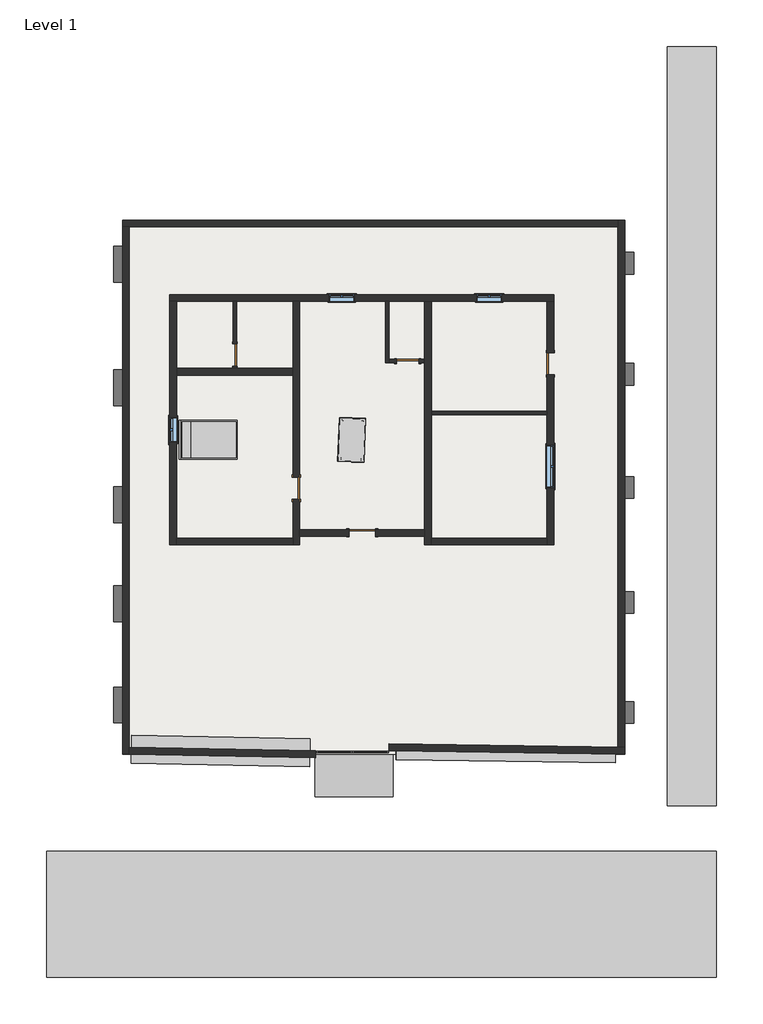
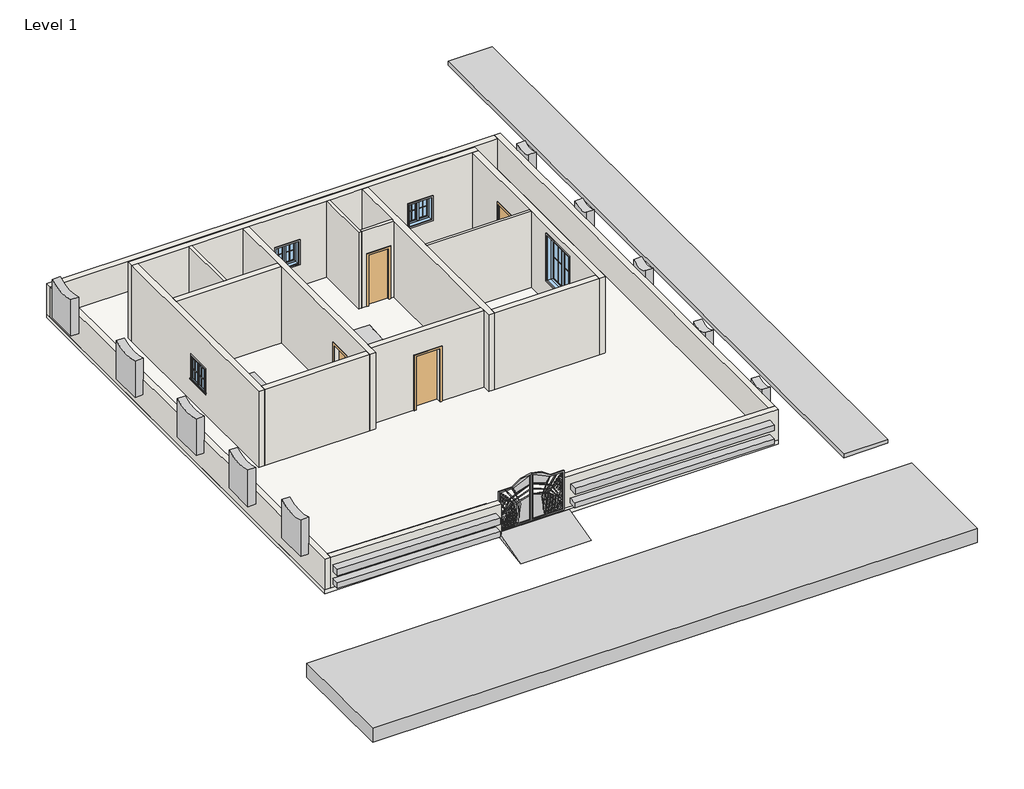
# One storey, incomplete: 24 proxies, 18 walls, 5 doors, 5 windows, 2 furniture elements, 1 slab.
"""IFC4 building model written with IfcOpenShell, lengths in millimetres."""

from ifc_helpers import new_model, si_unit, frame, origin, origin_with_axes, place, context, project, spatial, polyline, outline, extrude, faceted_brep, transform, mapped, element, save
from components import generic_models_6bc30956, generic_models_1_generic_models_1_9ac678b9, generic_models_2_generic_models_2_96ab2cd9, generic_models_4_generic_models_4_b5ce0ccc, generic_models_5_generic_models_5_faea7b41, generic_models_6_generic_models_6_873e410b, generic_models_7_generic_models_7_fbfc4c3c, generic_models_8_generic_models_8_d6955511, muntin_pattern_2x2_muntin_pattern_2x2_b3fe6957, muntin_pattern_2x2_muntin_pattern_2x2_3e0ecaf2, muntin_pattern_2x2_muntin_pattern_2x2_bff912c5, muntin_pattern_2x2_muntin_pattern_2x2_c2194282, trim_window_exterior_flat_with_sill_41619996, trim_window_exterior_flat_with_sill_e04b3088, trim_window_interior_flat_picture_frame_51c85655, trim_window_interior_flat_picture_frame_2a7685fe, door_d8f5dbb5, door_f2b275c1, door_85036156, door_0ca8825f, bed_17739_bed_17739_15c61121, dining_table_14755_dining_table_14755_d89cb775, window_aa618e30, window_339605e1, window_9ac97e1a

model = new_model("IFC4")

# Units and contexts
model_context = context("Model", 3, world=origin())
ifc_project = project(units=[si_unit("LENGTHUNIT", "METRE", prefix="MILLI")], contexts=[model_context])

# Site, building, storey
site = spatial("IfcSite", under=ifc_project)
building = spatial("IfcBuilding", under=site)
storey = spatial("IfcBuildingStorey", under=building, Name="Level 1", Elevation=0.0)

# Proxies
placement = place(None, origin())
generic_models_shape = generic_models_6bc30956(model_context)
element("IfcBuildingElementProxy", 1, Name="Generic Models", at=placement, inside=storey, context=model_context, shape_type="MappedRepresentation", body=[
    mapped(generic_models_shape, transform((-1300.5953031, -8339.7479738, 0.0), x_axis=(1.0, 0.0, 0.0), y_axis=(0.0, 1.0, 0.0), z_axis=(0.0, 0.0, 1.0))),
])
generic_models_1_generic_models_1_shape = generic_models_1_generic_models_1_9ac678b9(model_context)
element("IfcBuildingElementProxy", 2, Name="Generic Models 1 : Generic Models 1", ObjectType="Generic Models 1 : Generic Models 1", at=placement, inside=storey, context=model_context, shape_type="MappedRepresentation", body=[
    mapped(generic_models_1_generic_models_1_shape, transform((0.0, 0.0, 0.0), x_axis=(1.0, 0.0, 0.0), y_axis=(0.0, 1.0, 0.0), z_axis=(0.0, 0.0, 1.0))),
])
generic_models_2_generic_models_2_shape = generic_models_2_generic_models_2_96ab2cd9(model_context)
element("IfcBuildingElementProxy", 3, Name="Generic Models 2 : Generic Models 2", ObjectType="Generic Models 2 : Generic Models 2", at=placement, inside=storey, context=model_context, shape_type="MappedRepresentation", body=[
    mapped(generic_models_2_generic_models_2_shape, transform((0.0, 0.0, 0.0), x_axis=(1.0, 0.0, 0.0), y_axis=(0.0, 1.0, 0.0), z_axis=(0.0, 0.0, 1.0))),
])
generic_models_4_generic_models_4_shape = generic_models_4_generic_models_4_b5ce0ccc(model_context)
element("IfcBuildingElementProxy", 4, Name="Generic Models 4 : Generic Models 4", ObjectType="Generic Models 4 : Generic Models 4", at=placement, inside=storey, context=model_context, shape_type="MappedRepresentation", body=[
    mapped(generic_models_4_generic_models_4_shape, transform((0.0, 0.0, 0.0), x_axis=(1.0, 0.0, 0.0), y_axis=(0.0, 1.0, 0.0), z_axis=(0.0, 0.0, 1.0))),
])
generic_models_5_generic_models_5_shape = generic_models_5_generic_models_5_faea7b41(model_context)
element("IfcBuildingElementProxy", 5, Name="Generic Models 5 : Generic Models 5", ObjectType="Generic Models 5 : Generic Models 5", at=placement, inside=storey, context=model_context, shape_type="MappedRepresentation", body=[
    mapped(generic_models_5_generic_models_5_shape, transform((0.0, 0.0, 0.0), x_axis=(1.0, 0.0, 0.0), y_axis=(0.0, 1.0, 0.0), z_axis=(0.0, 0.0, 1.0))),
])
generic_models_6_generic_models_6_shape = generic_models_6_generic_models_6_873e410b(model_context)
element("IfcBuildingElementProxy", 6, Name="Generic Models 6 : Generic Models 6", ObjectType="Generic Models 6 : Generic Models 6", at=placement, inside=storey, context=model_context, shape_type="MappedRepresentation", body=[
    mapped(generic_models_6_generic_models_6_shape, transform((0.0, 0.0, 0.0), x_axis=(1.0, 0.0, 0.0), y_axis=(0.0, 1.0, 0.0), z_axis=(0.0, 0.0, 1.0))),
])
generic_models_7_generic_models_7_shape = generic_models_7_generic_models_7_fbfc4c3c(model_context)
element("IfcBuildingElementProxy", 7, Name="Generic Models 7 : Generic Models 7", ObjectType="Generic Models 7 : Generic Models 7", at=placement, inside=storey, context=model_context, shape_type="MappedRepresentation", body=[
    mapped(generic_models_7_generic_models_7_shape, transform((0.0, 0.0, 0.0), x_axis=(1.0, 0.0, 0.0), y_axis=(0.0, 1.0, 0.0), z_axis=(0.0, 0.0, 1.0))),
])
generic_models_8_generic_models_8_shape = generic_models_8_generic_models_8_d6955511(model_context)
element("IfcBuildingElementProxy", 8, Name="Generic Models 8 : Generic Models 8", ObjectType="Generic Models 8 : Generic Models 8", at=placement, inside=storey, context=model_context, shape_type="MappedRepresentation", body=[
    mapped(generic_models_8_generic_models_8_shape, transform((0.0, 0.0, 0.0), x_axis=(1.0, 0.0, 0.0), y_axis=(0.0, 1.0, 0.0), z_axis=(0.0, 0.0, 1.0))),
])
muntin_pattern_2x2_muntin_pattern_2x2_shape = muntin_pattern_2x2_muntin_pattern_2x2_b3fe6957(model_context)
element("IfcBuildingElementProxy", 9, Name="Muntin Pattern_2x2 : Muntin Pattern_2x2", ObjectType="Muntin Pattern_2x2 : Muntin Pattern_2x2", at=placement, inside=storey, context=model_context, shape_type="MappedRepresentation", body=[
    mapped(muntin_pattern_2x2_muntin_pattern_2x2_shape, transform((3164.7728376, 7227.4016064, 984.25), x_axis=(1.0, 0.0, 0.0), y_axis=(0.0, 1.0, 0.0), z_axis=(0.0, 0.0, 1.0))),
])
element("IfcBuildingElementProxy", 10, Name="Muntin Pattern_2x2 : Muntin Pattern_2x2", ObjectType="Muntin Pattern_2x2 : Muntin Pattern_2x2", at=placement, inside=storey, context=model_context, shape_type="MappedRepresentation", body=[
    mapped(muntin_pattern_2x2_muntin_pattern_2x2_shape, transform((-7515.213363, 2411.5985933, 984.25), x_axis=(0.0, 1.0, 0.0), y_axis=(-1.0, 0.0, 0.0), z_axis=(0.0, 0.0, 1.0))),
])
element("IfcBuildingElementProxy", 11, Name="Muntin Pattern_2x2 : Muntin Pattern_2x2", ObjectType="Muntin Pattern_2x2 : Muntin Pattern_2x2", at=placement, inside=storey, context=model_context, shape_type="MappedRepresentation", body=[
    mapped(muntin_pattern_2x2_muntin_pattern_2x2_shape, transform((-1868.0846872, 7227.4016064, 984.25), x_axis=(1.0, 0.0, 0.0), y_axis=(0.0, 1.0, 0.0), z_axis=(0.0, 0.0, 1.0))),
])
muntin_pattern_2x2_muntin_pattern_2x2_2_shape = muntin_pattern_2x2_muntin_pattern_2x2_3e0ecaf2(model_context)
element("IfcBuildingElementProxy", 12, Name="Muntin Pattern_2x2 : Muntin Pattern_2x2", ObjectType="Muntin Pattern_2x2 : Muntin Pattern_2x2", at=placement, inside=storey, context=model_context, shape_type="MappedRepresentation", body=[
    mapped(muntin_pattern_2x2_muntin_pattern_2x2_2_shape, transform((3593.3978376, 7227.4016064, 984.25), x_axis=(-1.0, 0.0, 0.0), y_axis=(0.0, -1.0, 0.0), z_axis=(0.0, 0.0, 1.0))),
])
element("IfcBuildingElementProxy", 13, Name="Muntin Pattern_2x2 : Muntin Pattern_2x2", ObjectType="Muntin Pattern_2x2 : Muntin Pattern_2x2", at=placement, inside=storey, context=model_context, shape_type="MappedRepresentation", body=[
    mapped(muntin_pattern_2x2_muntin_pattern_2x2_2_shape, transform((-7515.213363, 2840.2235933, 984.25), x_axis=(0.0, -1.0, 0.0), y_axis=(1.0, 0.0, 0.0), z_axis=(0.0, 0.0, 1.0))),
])
element("IfcBuildingElementProxy", 14, Name="Muntin Pattern_2x2 : Muntin Pattern_2x2", ObjectType="Muntin Pattern_2x2 : Muntin Pattern_2x2", at=placement, inside=storey, context=model_context, shape_type="MappedRepresentation", body=[
    mapped(muntin_pattern_2x2_muntin_pattern_2x2_2_shape, transform((-1439.4596872, 7227.4016064, 984.25), x_axis=(-1.0, 0.0, 0.0), y_axis=(0.0, -1.0, 0.0), z_axis=(0.0, 0.0, 1.0))),
])
muntin_pattern_2x2_muntin_pattern_2x2_3_shape = muntin_pattern_2x2_muntin_pattern_2x2_bff912c5(model_context)
element("IfcBuildingElementProxy", 15, Name="Muntin Pattern_2x2 : Muntin Pattern_2x2", ObjectType="Muntin Pattern_2x2 : Muntin Pattern_2x2", at=placement, inside=storey, context=model_context, shape_type="MappedRepresentation", body=[
    mapped(muntin_pattern_2x2_muntin_pattern_2x2_3_shape, transform((5572.923676, 1735.2928063, 984.25), x_axis=(0.0, -1.0, 0.0), y_axis=(1.0, 0.0, 0.0), z_axis=(0.0, 0.0, 1.0))),
])
muntin_pattern_2x2_muntin_pattern_2x2_4_shape = muntin_pattern_2x2_muntin_pattern_2x2_c2194282(model_context)
element("IfcBuildingElementProxy", 16, Name="Muntin Pattern_2x2 : Muntin Pattern_2x2", ObjectType="Muntin Pattern_2x2 : Muntin Pattern_2x2", at=placement, inside=storey, context=model_context, shape_type="MappedRepresentation", body=[
    mapped(muntin_pattern_2x2_muntin_pattern_2x2_4_shape, transform((5572.923676, 1014.5678063, 984.25), x_axis=(0.0, 1.0, 0.0), y_axis=(-1.0, 0.0, 0.0), z_axis=(0.0, 0.0, 1.0))),
])
trim_window_exterior_flat_with_sill_shape = trim_window_exterior_flat_with_sill_41619996(model_context)
element("IfcBuildingElementProxy", 17, Name="Trim-Window-Exterior-Flat : with Sill", ObjectType="Trim-Window-Exterior-Flat : with Sill", at=placement, inside=storey, context=model_context, shape_type="MappedRepresentation", body=[
    mapped(trim_window_exterior_flat_with_sill_shape, transform((3379.0853376, 7236.9266064, 1828.8), x_axis=(-1.0, 0.0, 0.0), y_axis=(0.0, 0.0, 1.0), z_axis=(0.0, 1.0, 0.0))),
])
element("IfcBuildingElementProxy", 18, Name="Trim-Window-Exterior-Flat : with Sill", ObjectType="Trim-Window-Exterior-Flat : with Sill", at=placement, inside=storey, context=model_context, shape_type="MappedRepresentation", body=[
    mapped(trim_window_exterior_flat_with_sill_shape, transform((-7524.738363, 2625.9110933, 1828.8), x_axis=(0.0, -1.0, 0.0), y_axis=(0.0, 0.0, 1.0), z_axis=(-1.0, 0.0, 0.0))),
])
element("IfcBuildingElementProxy", 19, Name="Trim-Window-Exterior-Flat : with Sill", ObjectType="Trim-Window-Exterior-Flat : with Sill", at=placement, inside=storey, context=model_context, shape_type="MappedRepresentation", body=[
    mapped(trim_window_exterior_flat_with_sill_shape, transform((-1653.7721872, 7236.9266064, 1828.8), x_axis=(-1.0, 0.0, 0.0), y_axis=(0.0, 0.0, 1.0), z_axis=(0.0, 1.0, 0.0))),
])
trim_window_exterior_flat_with_sill_2_shape = trim_window_exterior_flat_with_sill_e04b3088(model_context)
element("IfcBuildingElementProxy", 20, Name="Trim-Window-Exterior-Flat : with Sill", ObjectType="Trim-Window-Exterior-Flat : with Sill", at=placement, inside=storey, context=model_context, shape_type="MappedRepresentation", body=[
    mapped(trim_window_exterior_flat_with_sill_2_shape, transform((5582.448676, 1374.9303063, 2743.2), x_axis=(0.0, 1.0, 0.0), y_axis=(0.0, 0.0, 1.0), z_axis=(1.0, 0.0, 0.0))),
])
trim_window_interior_flat_picture_frame_shape = trim_window_interior_flat_picture_frame_51c85655(model_context)
element("IfcBuildingElementProxy", 21, Name="Trim-Window-Interior-Flat : Picture Frame", ObjectType="Trim-Window-Interior-Flat : Picture Frame", at=placement, inside=storey, context=model_context, shape_type="MappedRepresentation", body=[
    mapped(trim_window_interior_flat_picture_frame_shape, transform((3379.0853376, 7008.3266064, 1828.8), x_axis=(1.0, 0.0, 0.0), y_axis=(0.0, 0.0, 1.0), z_axis=(0.0, -1.0, 0.0))),
])
element("IfcBuildingElementProxy", 22, Name="Trim-Window-Interior-Flat : Picture Frame", ObjectType="Trim-Window-Interior-Flat : Picture Frame", at=placement, inside=storey, context=model_context, shape_type="MappedRepresentation", body=[
    mapped(trim_window_interior_flat_picture_frame_shape, transform((-7296.138363, 2625.9110933, 1828.8), x_axis=(0.0, 1.0, 0.0), y_axis=(0.0, 0.0, 1.0), z_axis=(1.0, 0.0, 0.0))),
])
element("IfcBuildingElementProxy", 23, Name="Trim-Window-Interior-Flat : Picture Frame", ObjectType="Trim-Window-Interior-Flat : Picture Frame", at=placement, inside=storey, context=model_context, shape_type="MappedRepresentation", body=[
    mapped(trim_window_interior_flat_picture_frame_shape, transform((-1653.7721872, 7008.3266064, 1828.8), x_axis=(1.0, 0.0, 0.0), y_axis=(0.0, 0.0, 1.0), z_axis=(0.0, -1.0, 0.0))),
])
trim_window_interior_flat_picture_frame_2_shape = trim_window_interior_flat_picture_frame_2a7685fe(model_context)
element("IfcBuildingElementProxy", 24, Name="Trim-Window-Interior-Flat : Picture Frame", ObjectType="Trim-Window-Interior-Flat : Picture Frame", at=placement, inside=storey, context=model_context, shape_type="MappedRepresentation", body=[
    mapped(trim_window_interior_flat_picture_frame_2_shape, transform((5353.848676, 1374.9303063, 2743.2), x_axis=(0.0, -1.0, 0.0), y_axis=(0.0, 0.0, 1.0), z_axis=(-1.0, 0.0, 0.0))),
])

# Doors
door_shape = door_d8f5dbb5(model_context)
element("IfcDoor", 25, ObjectType="Single-Flush : 30\" x 80\"", at=placement, inside=storey, context=model_context, shape_type="MappedRepresentation", body=[
    mapped(door_shape, transform((-5307.8080357, 5179.2254479, 0.0), x_axis=(0.0, -1.0, 0.0), y_axis=(1.0, 0.0, 0.0), z_axis=(0.0, 0.0, 1.0))),
])
door_2_shape = door_f2b275c1(model_context)
element("IfcDoor", 26, ObjectType="Single-Flush : 30\" x 80\"", at=placement, inside=storey, context=model_context, shape_type="MappedRepresentation", body=[
    mapped(door_2_shape, transform((594.788348, 4969.6493483, 0.0), x_axis=(-1.0, 0.0, 0.0), y_axis=(0.0, -1.0, 0.0), z_axis=(0.0, 0.0, 1.0))),
])
door_3_shape = door_85036156(model_context)
element("IfcDoor", 27, ObjectType="Single-Flush : 30\" x 80\"", at=placement, inside=storey, context=model_context, shape_type="MappedRepresentation", body=[
    mapped(door_3_shape, transform((5468.148676, 4880.1303063, 0.0), x_axis=(0.0, -1.0, 0.0), y_axis=(1.0, 0.0, 0.0), z_axis=(0.0, 0.0, 1.0))),
])
element("IfcDoor", 28, ObjectType="Single-Flush : 30\" x 80\"", at=placement, inside=storey, context=model_context, shape_type="MappedRepresentation", body=[
    mapped(door_3_shape, transform((-3207.0990712, 633.8093082, 0.0), x_axis=(0.0, 1.0, 0.0), y_axis=(-1.0, 0.0, 0.0), z_axis=(0.0, 0.0, 1.0))),
])
door_4_shape = door_0ca8825f(model_context)
element("IfcDoor", 29, ObjectType="Single-Flush : 36\" x 84\"", at=placement, inside=storey, context=model_context, shape_type="MappedRepresentation", body=[
    mapped(door_4_shape, transform((-958.538536, -890.1906918, 0.0), x_axis=(1.0, 0.0, 0.0), y_axis=(0.0, 1.0, 0.0), z_axis=(0.0, 0.0, 1.0))),
])

# Furniture
bed_17739_bed_17739_shape = bed_17739_bed_17739_15c61121(model_context)
element("IfcFurniture", 30, ObjectType="Bed_17739 : Bed_17739", at=placement, inside=storey, context=model_context, shape_type="MappedRepresentation", body=[
    mapped(bed_17739_bed_17739_shape, transform((-6191.238363, 2289.3303063, 0.0), x_axis=(0.0, 1.0, 0.0), y_axis=(-1.0, 0.0, 0.0), z_axis=(0.0, 0.0, 1.0))),
])
dining_table_14755_dining_table_14755_shape = dining_table_14755_dining_table_14755_d89cb775(model_context)
element("IfcFurniture", 31, ObjectType="Dining_table_14755 : Dining_table_14755", at=placement, inside=storey, context=model_context, shape_type="MappedRepresentation", body=[
    mapped(dining_table_14755_dining_table_14755_shape, transform((-893.6639349, 1513.0244832, 0.0), x_axis=(0.03701166050986843, 0.9993148337667677, 0.0), y_axis=(-0.9993148337667677, 0.03701166050986843, 0.0), z_axis=(0.0, 0.0, 1.0))),
])

# Slab
element("IfcSlab", 32, ObjectType="Generic - 12\"", at=placement, inside=storey, context=model_context, shape_type="SweptSolid", body=[
    extrude(outline(polyline([(8003.5487756, 9776.8020262), (8003.5487756, -8436.6963345), (-9141.4512244, -8436.6963345), (-9141.4512244, 9776.8020262), (8003.5487756, 9776.8020262)])), frame((0.0, 0.0, -152.4), z_axis=(0.0, 0.0, 1.0), x_axis=(1.0, 0.0, 0.0)), (0.0, 0.0, 1.0), 152.4),
])

# Walls
element("IfcWall", 33, ObjectType="WALL4.5\"", at=placement, inside=storey, context=model_context, shape_type="SweptSolid", body=[
    extrude(outline(polyline([(4798.2254479, 2032.0), (4798.2254479, 0.0), (4722.0254479, 0.0), (4722.0254479, 3048.0), (7008.3266064, 3048.0), (7008.3266064, 0.0), (5560.2254479, 0.0), (5560.2254479, 2032.0), (4798.2254479, 2032.0)])), frame((-5364.9580357, 0.0, 0.0), z_axis=(1.0, 0.0, 0.0), x_axis=(0.0, 1.0, 0.0)), (0.0, 0.0, 1.0), 114.3),
])
element("IfcWall", 34, ObjectType="WALL4.5\"", at=placement, inside=storey, context=model_context, shape_type="Brep", body=[
    faceted_brep([(-157.5953031, 7008.3266064, 0.0), (-157.5953031, 4912.4993483, 0.0), (-157.5953031, 4912.4993483, 3048.0), (-157.5953031, 7008.3266064, 3048.0), (-43.2953031, 7008.3266064, 0.0), (-43.2953031, 7008.3266064, 3048.0), (-43.2953031, 5026.7993483, 3048.0), (-43.2953031, 4912.4993483, 3048.0), (-43.2953031, 4912.4993483, 0.0), (-43.2953031, 5026.7993483, 0.0)], [[[0, 1, 2, 3]], [[4, 5, 6, 7, 8, 9]], [[1, 0, 4, 9, 8]], [[0, 3, 5, 4]], [[2, 1, 8, 7]], [[3, 2, 7, 6, 5]]]),
])
element("IfcWall", 35, ObjectType="WALL4.5\"", at=placement, inside=storey, context=model_context, shape_type="SweptSolid", body=[
    extrude(outline(polyline([(0.0, -43.2953031), (0.0, 213.788348), (2032.0, 213.788348), (2032.0, 975.788348), (0.0, 975.788348), (0.0, 1175.7219991), (3048.0, 1175.7219991), (3048.0, -43.2953031), (0.0, -43.2953031)])), frame((0.0, 4912.4993483, 0.0), z_axis=(0.0, 1.0, 0.0), x_axis=(0.0, 0.0, 1.0)), (0.0, 0.0, 1.0), 114.3),
])
element("IfcWall", 36, ObjectType="WALL4.5\"", at=placement, inside=storey, context=model_context, shape_type="SweptSolid", body=[
    extrude(outline(polyline([(1404.3219991, 3260.8803063), (5353.848676, 3260.8803063), (5353.848676, 3146.5803063), (1404.3219991, 3146.5803063), (1404.3219991, 3260.8803063)])), origin_with_axes(), (0.0, 0.0, 1.0), 3048.0),
])
element("IfcWall", 37, ObjectType="WALL9\"", at=placement, inside=storey, context=model_context, shape_type="Brep", body=[
    faceted_brep([(-7524.738363, 7008.3266064, 0.0), (-7296.138363, 7008.3266064, 0.0), (-5364.9580357, 7008.3266064, 0.0), (-5250.6580357, 7008.3266064, 0.0), (-3321.3990712, 7008.3266064, 0.0), (-3092.7990712, 7008.3266064, 0.0), (-157.5953031, 7008.3266064, 0.0), (-43.2953031, 7008.3266064, 0.0), (1175.7219991, 7008.3266064, 0.0), (1404.3219991, 7008.3266064, 0.0), (5353.848676, 7008.3266064, 0.0), (5582.448676, 7008.3266064, 0.0), (5582.448676, 7008.3266064, 3048.0), (5353.848676, 7008.3266064, 3048.0), (1404.3219991, 7008.3266064, 3048.0), (1175.7219991, 7008.3266064, 3048.0), (-43.2953031, 7008.3266064, 3048.0), (-157.5953031, 7008.3266064, 3048.0), (-3092.7990712, 7008.3266064, 3048.0), (-3321.3990712, 7008.3266064, 3048.0), (-5250.6580357, 7008.3266064, 3048.0), (-5364.9580357, 7008.3266064, 3048.0), (-7296.138363, 7008.3266064, 3048.0), (-7524.738363, 7008.3266064, 3048.0), (-4054.2535534, 7008.3266064, 787.4), (-4054.2535534, 7008.3266064, 177.8), (-4460.6535534, 7008.3266064, 177.8), (-4460.6535534, 7008.3266064, 787.4), (3810.8853376, 7008.3266064, 1828.8), (3810.8853376, 7008.3266064, 914.4), (2947.2853376, 7008.3266064, 914.4), (2947.2853376, 7008.3266064, 1828.8), (-1221.9721872, 7008.3266064, 1828.8), (-1221.9721872, 7008.3266064, 914.4), (-2085.5721872, 7008.3266064, 914.4), (-2085.5721872, 7008.3266064, 1828.8), (-7524.738363, 7236.9266064, 0.0), (-7524.738363, 7236.9266064, 3048.0), (5582.448676, 7236.9266064, 3048.0), (5582.448676, 7236.9266064, 0.0), (-4054.2535534, 7236.9266064, 787.4), (-4460.6535534, 7236.9266064, 787.4), (-4460.6535534, 7236.9266064, 177.8), (-4054.2535534, 7236.9266064, 177.8), (3810.8853376, 7236.9266064, 1828.8), (2947.2853376, 7236.9266064, 1828.8), (2947.2853376, 7236.9266064, 914.4), (3810.8853376, 7236.9266064, 914.4), (-1221.9721872, 7236.9266064, 1828.8), (-2085.5721872, 7236.9266064, 1828.8), (-2085.5721872, 7236.9266064, 914.4), (-1221.9721872, 7236.9266064, 914.4)], [[[0, 1, 2, 3, 4, 5, 6, 7, 8, 9, 10, 11, 12, 13, 14, 15, 16, 17, 18, 19, 20, 21, 22, 23], [24, 25, 26, 27], [28, 29, 30, 31], [32, 33, 34, 35]], [[36, 37, 38, 39], [40, 41, 42, 43], [44, 45, 46, 47], [48, 49, 50, 51]], [[11, 10, 9, 8, 7, 6, 5, 4, 3, 2, 1, 0, 36, 39]], [[12, 11, 39, 38]], [[0, 23, 37, 36]], [[23, 22, 21, 20, 19, 18, 17, 16, 15, 14, 13, 12, 38, 37]], [[25, 24, 40, 43]], [[26, 25, 43, 42]], [[27, 26, 42, 41]], [[24, 27, 41, 40]], [[29, 28, 44, 47]], [[30, 29, 47, 46]], [[31, 30, 46, 45]], [[28, 31, 45, 44]], [[33, 32, 48, 51]], [[34, 33, 51, 50]], [[35, 34, 50, 49]], [[32, 35, 49, 48]]]),
])
element("IfcWall", 38, ObjectType="WALL9\"", at=placement, inside=storey, context=model_context, shape_type="Brep", body=[
    faceted_brep([(5353.848676, 4499.1303063, 2032.0), (5353.848676, 4499.1303063, 0.0), (5353.848676, 3260.8803063, 0.0), (5353.848676, 3146.5803063, 0.0), (5353.848676, -1070.2868249, 0.0), (5353.848676, -1298.8868249, 0.0), (5353.848676, -1298.8868249, 3048.0), (5353.848676, -1070.2868249, 3048.0), (5353.848676, 3146.5803063, 3048.0), (5353.848676, 3260.8803063, 3048.0), (5353.848676, 7008.3266064, 3048.0), (5353.848676, 7008.3266064, 0.0), (5353.848676, 5261.1303063, 0.0), (5353.848676, 5261.1303063, 2032.0), (5353.848676, 651.0303063, 2743.2), (5353.848676, 651.0303063, 914.4), (5353.848676, 2098.8303063, 914.4), (5353.848676, 2098.8303063, 2743.2), (5582.448676, -1298.8868249, 0.0), (5582.448676, 4499.1303063, 0.0), (5582.448676, 4499.1303063, 2032.0), (5582.448676, 5261.1303063, 2032.0), (5582.448676, 5261.1303063, 0.0), (5582.448676, 7008.3266064, 0.0), (5582.448676, 7008.3266064, 3048.0), (5582.448676, -1298.8868249, 3048.0), (5582.448676, 651.0303063, 2743.2), (5582.448676, 2098.8303063, 2743.2), (5582.448676, 2098.8303063, 914.4), (5582.448676, 651.0303063, 914.4)], [[[0, 1, 2, 3, 4, 5, 6, 7, 8, 9, 10, 11, 12, 13], [14, 15, 16, 17]], [[18, 19, 20, 21, 22, 23, 24, 25], [26, 27, 28, 29]], [[12, 11, 23, 22]], [[5, 4, 3, 2, 1, 19, 18]], [[11, 10, 24, 23]], [[6, 5, 18, 25]], [[20, 19, 1, 0]], [[21, 20, 0, 13]], [[22, 21, 13, 12]], [[10, 9, 8, 7, 6, 25, 24]], [[15, 14, 26, 29]], [[16, 15, 29, 28]], [[17, 16, 28, 27]], [[14, 17, 27, 26]]]),
])
element("IfcWall", 39, ObjectType="WALL9\"", at=placement, inside=storey, context=model_context, shape_type="Brep", body=[
    faceted_brep([(-7296.138363, -1298.8868249, 0.0), (-7296.138363, -1070.2868249, 0.0), (-7296.138363, 4492.8110933, 0.0), (-7296.138363, 4721.4110933, 0.0), (-7296.138363, 7008.3266064, 0.0), (-7296.138363, 7008.3266064, 3048.0), (-7296.138363, 4721.4110933, 3048.0), (-7296.138363, 4492.8110933, 3048.0), (-7296.138363, -1070.2868249, 3048.0), (-7296.138363, -1298.8868249, 3048.0), (-7296.138363, 3057.7110933, 1828.8), (-7296.138363, 3057.7110933, 914.4), (-7296.138363, 2194.1110933, 914.4), (-7296.138363, 2194.1110933, 1828.8), (-7524.738363, -1298.8868249, 0.0), (-7524.738363, -1298.8868249, 3048.0), (-7524.738363, 7008.3266064, 3048.0), (-7524.738363, 7008.3266064, 0.0), (-7524.738363, 3057.7110933, 1828.8), (-7524.738363, 2194.1110933, 1828.8), (-7524.738363, 2194.1110933, 914.4), (-7524.738363, 3057.7110933, 914.4)], [[[0, 1, 2, 3, 4, 5, 6, 7, 8, 9], [10, 11, 12, 13]], [[14, 15, 16, 17], [18, 19, 20, 21]], [[4, 3, 2, 1, 0, 14, 17]], [[5, 4, 17, 16]], [[0, 9, 15, 14]], [[9, 8, 7, 6, 5, 16, 15]], [[11, 10, 18, 21]], [[12, 11, 21, 20]], [[13, 12, 20, 19]], [[10, 13, 19, 18]]]),
])
element("IfcWall", 40, ObjectType="WALL9\"", at=placement, inside=storey, context=model_context, shape_type="Brep", body=[
    faceted_brep([(-3321.3990712, 7008.3266064, 0.0), (-3321.3990712, 4721.4110933, 0.0), (-3321.3990712, 4492.8110933, 0.0), (-3321.3990712, 1014.8093082, 0.0), (-3321.3990712, 1014.8093082, 2032.0), (-3321.3990712, 252.8093082, 2032.0), (-3321.3990712, 252.8093082, 0.0), (-3321.3990712, -1070.2868249, 0.0), (-3321.3990712, -1298.8868249, 0.0), (-3321.3990712, -1298.8868249, 3048.0), (-3321.3990712, -1070.2868249, 3048.0), (-3321.3990712, 4492.8110933, 3048.0), (-3321.3990712, 4721.4110933, 3048.0), (-3321.3990712, 7008.3266064, 3048.0), (-3092.7990712, 1014.8093082, 2032.0), (-3092.7990712, 1014.8093082, 0.0), (-3092.7990712, 7008.3266064, 0.0), (-3092.7990712, 7008.3266064, 3048.0), (-3092.7990712, -775.8906918, 3048.0), (-3092.7990712, -1004.4906918, 3048.0), (-3092.7990712, -1298.8868249, 3048.0), (-3092.7990712, -1298.8868249, 0.0), (-3092.7990712, -1004.4906918, 0.0), (-3092.7990712, -775.8906918, 0.0), (-3092.7990712, 252.8093082, 0.0), (-3092.7990712, 252.8093082, 2032.0)], [[[0, 1, 2, 3, 4, 5, 6, 7, 8, 9, 10, 11, 12, 13]], [[14, 15, 16, 17, 18, 19, 20, 21, 22, 23, 24, 25]], [[16, 15, 3, 2, 1, 0]], [[24, 23, 22, 21, 8, 7, 6]], [[0, 13, 17, 16]], [[9, 8, 21, 20]], [[4, 3, 15, 14]], [[5, 4, 14, 25]], [[6, 5, 25, 24]], [[13, 12, 11, 10, 9, 20, 19, 18, 17]]]),
])
element("IfcWall", 41, ObjectType="WALL9\"", at=placement, inside=storey, context=model_context, shape_type="Brep", body=[
    faceted_brep([(1175.7219991, 7008.3266064, 0.0), (1175.7219991, 5026.7993483, 0.0), (1175.7219991, 4912.4993483, 0.0), (1175.7219991, -775.8906918, 0.0), (1175.7219991, -1004.4906918, 0.0), (1175.7219991, -1298.8868249, 0.0), (1175.7219991, -1298.8868249, 3048.0), (1175.7219991, -1004.4906918, 3048.0), (1175.7219991, -775.8906918, 3048.0), (1175.7219991, 4912.4993483, 3048.0), (1175.7219991, 5026.7993483, 3048.0), (1175.7219991, 7008.3266064, 3048.0), (1404.3219991, 7008.3266064, 0.0), (1404.3219991, 7008.3266064, 3048.0), (1404.3219991, 3260.8803063, 3048.0), (1404.3219991, 3146.5803063, 3048.0), (1404.3219991, -1070.2868249, 3048.0), (1404.3219991, -1298.8868249, 3048.0), (1404.3219991, -1298.8868249, 0.0), (1404.3219991, -1070.2868249, 0.0), (1404.3219991, 3146.5803063, 0.0), (1404.3219991, 3260.8803063, 0.0)], [[[0, 1, 2, 3, 4, 5, 6, 7, 8, 9, 10, 11]], [[12, 13, 14, 15, 16, 17, 18, 19, 20, 21]], [[5, 4, 3, 2, 1, 0, 12, 21, 20, 19, 18]], [[0, 11, 13, 12]], [[6, 5, 18, 17]], [[11, 10, 9, 8, 7, 6, 17, 16, 15, 14, 13]]]),
])
element("IfcWall", 42, ObjectType="WALL9\"", at=placement, inside=storey, context=model_context, shape_type="SweptSolid", body=[
    extrude(outline(polyline([(-3321.3990712, -1298.8868249), (-7296.138363, -1298.8868249), (-7296.138363, -1070.2868249), (-3321.3990712, -1070.2868249), (-3321.3990712, -1298.8868249)])), origin_with_axes(), (0.0, 0.0, 1.0), 3048.0),
])
element("IfcWall", 43, ObjectType="WALL9\"", at=placement, inside=storey, context=model_context, shape_type="SweptSolid", body=[
    extrude(outline(polyline([(5353.848676, -1298.8868249), (1404.3219991, -1298.8868249), (1404.3219991, -1070.2868249), (5353.848676, -1070.2868249), (5353.848676, -1298.8868249)])), origin_with_axes(), (0.0, 0.0, 1.0), 3048.0),
])
element("IfcWall", 44, ObjectType="WALL9\"", at=placement, inside=storey, context=model_context, shape_type="SweptSolid", body=[
    extrude(outline(polyline([(2133.6, -501.338536), (0.0, -501.338536), (0.0, 1175.7219991), (3048.0, 1175.7219991), (3048.0, -3092.7990712), (0.0, -3092.7990712), (0.0, -1415.738536), (2133.6, -1415.738536), (2133.6, -501.338536)])), frame((0.0, -1004.4906918, 0.0), z_axis=(0.0, 1.0, 0.0), x_axis=(0.0, 0.0, 1.0)), (0.0, 0.0, 1.0), 228.6),
])
element("IfcWall", 45, ObjectType="WALL9\"", at=placement, inside=storey, context=model_context, shape_type="SweptSolid", body=[
    extrude(outline(polyline([(-3321.3990712, 4492.8110933), (-7296.138363, 4492.8110933), (-7296.138363, 4721.4110933), (-3321.3990712, 4721.4110933), (-3321.3990712, 4492.8110933)])), origin_with_axes(), (0.0, 0.0, 1.0), 3048.0),
])
element("IfcWall", 46, ObjectType="WALL9\"", at=placement, inside=storey, context=model_context, shape_type="Brep", body=[
    faceted_brep([(-9141.4512244, 9548.2020262, 0.0), (-8912.8512244, 9548.2020262, 0.0), (7774.9487756, 9548.2020262, 0.0), (7774.9487756, 9548.2020262, 1219.2), (-8912.8512244, 9548.2020262, 1219.2), (-9141.4512244, 9548.2020262, 1219.2), (-9141.4512244, 9776.8020262, 0.0), (-9141.4512244, 9776.8020262, 1219.2), (7774.9487756, 9776.8020262, 1219.2), (7774.9487756, 9776.8020262, 0.0)], [[[0, 1, 2, 3, 4, 5]], [[6, 7, 8, 9]], [[2, 1, 0, 6, 9]], [[5, 4, 3, 8, 7]], [[0, 5, 7, 6]], [[3, 2, 9, 8]]]),
])
element("IfcWall", 47, ObjectType="WALL9\"", at=placement, inside=storey, context=model_context, shape_type="Brep", body=[
    faceted_brep([(-8912.8512244, -8437.2801707, 0.0), (-8912.8512244, -8208.6363404, 0.0), (-8912.8512244, 9548.2020262, 0.0), (-8912.8512244, 9548.2020262, 1219.2), (-8912.8512244, -8208.6363404, 1219.2), (-8912.8512244, -8437.2801707, 1219.2), (-9141.4512244, -8432.8034376, 0.0), (-9141.4512244, -8432.8034376, 1219.2), (-9141.4512244, 9548.2020262, 1219.2), (-9141.4512244, 9548.2020262, 0.0)], [[[0, 1, 2, 3, 4, 5]], [[6, 7, 8, 9]], [[2, 1, 0, 6, 9]], [[5, 4, 3, 8, 7]], [[0, 5, 7, 6]], [[3, 2, 9, 8]]]),
])
element("IfcWall", 48, ObjectType="WALL9\"", at=placement, inside=storey, context=model_context, shape_type="Brep", body=[
    faceted_brep([(8003.5487756, -8208.0718234, 0.0), (7774.9487756, -8204.7241243, 0.0), (-34.7015963, -8090.3568462, 0.0), (-34.7015963, -8090.3568462, 1219.2), (7774.9487756, -8204.7241243, 1219.2), (8003.5487756, -8208.0718234, 1219.2), (8003.5487756, -8436.6963345, 0.0), (8003.5487756, -8436.6963345, 1219.2), (-38.0489366, -8318.9323377, 1219.2), (-38.0489366, -8318.9323377, 0.0)], [[[0, 1, 2, 3, 4, 5]], [[6, 7, 8, 9]], [[2, 1, 0, 6, 9]], [[3, 2, 9, 8]], [[5, 4, 3, 8, 7]], [[0, 5, 7, 6]]]),
])
element("IfcWall", 49, ObjectType="WALL9\"", at=placement, inside=storey, context=model_context, shape_type="Brep", body=[
    faceted_brep([(7774.9487756, 9776.8020262, 0.0), (7774.9487756, 9548.2020262, 0.0), (7774.9487756, -8204.7241243, 0.0), (7774.9487756, -8204.7241243, 1219.2), (7774.9487756, 9548.2020262, 1219.2), (7774.9487756, 9776.8020262, 1219.2), (8003.5487756, 9776.8020262, 0.0), (8003.5487756, 9776.8020262, 1219.2), (8003.5487756, -8208.0718234, 1219.2), (8003.5487756, -8208.0718234, 0.0)], [[[0, 1, 2, 3, 4, 5]], [[6, 7, 8, 9]], [[2, 1, 0, 6, 9]], [[5, 4, 3, 8, 7]], [[0, 5, 7, 6]], [[3, 2, 9, 8]]]),
])
element("IfcWall", 50, ObjectType="WALL9\"", at=placement, inside=storey, context=model_context, shape_type="SweptSolid", body=[
    extrude(outline(polyline([(-8912.8512244, -8208.6363404), (-2542.0203031, -8333.3979738), (-2546.496178, -8561.9541519), (-8912.8512244, -8437.2801707), (-8912.8512244, -8208.6363404)])), origin_with_axes(), (0.0, 0.0, 1.0), 1219.2),
])

# Windows
window_shape = window_aa618e30(model_context)
element("IfcWindow", 51, ObjectType="Fixed : 16\" x 24\"", at=placement, inside=storey, context=model_context, shape_type="MappedRepresentation", body=[
    mapped(window_shape, transform((-4219.3535534, 7122.6266064, -736.6), x_axis=(1.0, 0.0, 0.0), y_axis=(0.0, 1.0, 0.0), z_axis=(0.0, 0.0, 1.0))),
])
window_2_shape = window_339605e1(model_context)
element("IfcWindow", 52, ObjectType="Window-Casement-Double : 34\" x 36\"", at=placement, inside=storey, context=model_context, shape_type="MappedRepresentation", body=[
    mapped(window_2_shape, transform((3379.0853376, 7122.6266064, 0.0), x_axis=(1.0, 0.0, 0.0), y_axis=(0.0, 1.0, 0.0), z_axis=(0.0, 0.0, 1.0))),
])
element("IfcWindow", 53, ObjectType="Window-Casement-Double : 34\" x 36\"", at=placement, inside=storey, context=model_context, shape_type="MappedRepresentation", body=[
    mapped(window_2_shape, transform((-7410.438363, 2625.9110933, 0.0), x_axis=(0.0, 1.0, 0.0), y_axis=(-1.0, 0.0, 0.0), z_axis=(0.0, 0.0, 1.0))),
])
element("IfcWindow", 54, ObjectType="Window-Casement-Double : 34\" x 36\"", at=placement, inside=storey, context=model_context, shape_type="MappedRepresentation", body=[
    mapped(window_2_shape, transform((-1653.7721872, 7122.6266064, 0.0), x_axis=(1.0, 0.0, 0.0), y_axis=(0.0, 1.0, 0.0), z_axis=(0.0, 0.0, 1.0))),
])
window_3_shape = window_9ac97e1a(model_context)
element("IfcWindow", 55, ObjectType="Window-Casement-Double : 57\" x 72\"", at=placement, inside=storey, context=model_context, shape_type="MappedRepresentation", body=[
    mapped(window_3_shape, transform((5468.148676, 1374.9303063, 0.0), x_axis=(0.0, -1.0, 0.0), y_axis=(1.0, 0.0, 0.0), z_axis=(0.0, 0.0, 1.0))),
])

save(model, "model.ifc")

# Revit data of these elements
# Type
#   m.s. sheet = none
#   2" x2" pipe = none
#   1"x1"pipe = none
#   Default Elevation = 0
# Type "Muntin Pattern_2x2 : Muntin Pattern_2x2"
#   Width [instance default] = 4' - 0"
#   Thickness = 0' - 0 1/2"
#   Height [instance default] = 4' - 0"
#   Distance = 0' - 0 3/4"
#   Interior Material [instance default] = none
#   Exterior Material [instance default] = none
#   Default Elevation = 0
# Type "Trim-Window-Exterior-Flat : with Sill"
#   Trim Width = 0' - 2 1/4"
#   Trim Thickness_Picture Frame = 0' - 1 1/4"
#   Trim Thickness_with Sill = 0' - 0 3/4"
#   Sill Thickness = 0' - 1 1/4"
#   Opening Width [instance default] = 2' - 0"
#   Opening Height [instance default] = 3' - 0"
#   Default Elevation = 4' - 0"
#   Sill = yes
#   Picture Frame = no
#   Trim Material [instance default] = none
# Type "Trim-Window-Interior-Flat : Picture Frame"
#   Trim Thickness_Picture Frame = 0' - 1 1/4"
#   Trim Width = 0' - 2 1/4"
#   Trim Thickness_with Sill = 0' - 0 3/4"
#   Sill Thickness = 0' - 1 1/4"
#   Opening Width [instance default] = 2' - 0"
#   Opening Height [instance default] = 3' - 0"
#   Default Elevation = 4' - 0"
#   Sill = no
#   Picture Frame = yes
#   Trim Material [instance default] = none
# Type "Single-Flush : 30\" x 80\""
#   Type Mark = "5"
#   Construction Type Id = "MDOOR"
#   Assembly Code = "C1020"
#   Analytic Construction = "Metal"
#   Thickness = 0' - 2"
#   Heat Transfer Coefficient (U) = 0.651978 BTU/(h·ft²·°F)
#   Height = 6' - 8"
#   Trim Projection Ext = 0' - 1"
#   Trim Projection Int = 0' - 1"
#   Trim Width = 0' - 3"
#   Width = 2' - 6"
#   Define Thermal Properties by = 1
#   Define Thermal Properties by = 1
#   Door Material = Door - Panel
#   Frame Material = Door - Frame
#   Visual Light Transmittance = 0
#   Solar Heat Gain Coefficient = 0
#   Function = (empty or 0)
#   Wall Closure = (empty or 0)
# Type "Single-Flush : 36\" x 84\""
#   Type Mark = "1"
#   Construction Type Id = "MDOOR"
#   Assembly Code = "C1020"
#   Analytic Construction = "Metal"
#   Thickness = 0' - 2"
#   Heat Transfer Coefficient (U) = 0.651978 BTU/(h·ft²·°F)
#   Height = 7' - 0"
#   Trim Projection Ext = 0' - 1"
#   Trim Projection Int = 0' - 1"
#   Trim Width = 0' - 3"
#   Width = 3' - 0"
#   Define Thermal Properties by = 1
#   Define Thermal Properties by = 1
#   Door Material = Door - Panel
#   Frame Material = Door - Frame
#   Visual Light Transmittance = 0
#   Solar Heat Gain Coefficient = 0
#   Function = (empty or 0)
#   Wall Closure = (empty or 0)
# Type "Bed_17739 : Bed_17739"
#   Default Elevation = 0
# Type "Dining_table_14755 : Dining_table_14755"
#   Lengte [instance default] = 4' - 11.05512"
#   Breedte [instance default] = 2' - 11.43307"
#   Tafelblad = none
#   Poten = none
#   Default Elevation = 0
# Type "Generic - 12\""
#   Assembly Code = "B1010"
#   Function = 0
#   Layers, outside or top first: 0' - 6" no material (function 1)
# Type "WALL4.5\""
#   Assembly Code = "B2010"
#   Layers, outside or top first: 0' - 4 1/2" no material (function 1)
# Type "WALL9\""
#   Assembly Code = "B2010"
#   Layers, outside or top first: 0' - 9" no material (function 1)
# Type "Fixed : 16\" x 24\""
#   Type Mark = "4"
#   Construction Type Id = "GSP4R"
#   Assembly Code = "B2020100"
#   Analytic Construction = "1/8 in Pilkington single glazing"
#   Visual Light Transmittance = 0.9
#   Solar Heat Gain Coefficient = 0.78
#   Heat Transfer Coefficient (U) = 0.6496 BTU/(h·ft²·°F)
#   Height = 2' - 0"
#   Default Sill Height = 3' - 0"
#   Width = 1' - 4"
#   Window Inset = 0' - 0 3/4"
#   Define Thermal Properties by = 1
#   Define Thermal Properties by = 1
#   Glass Pane Material = Glass
#   Sash Material = Sash
#   Wall Closure = (empty or 0)
# Type "Window-Casement-Double : 34\" x 36\""
#   Type Mark = "14"
#   Fire Rating = "0.5h"
#   Assembly Code = "B2020100"
#   Analytic Construction = "Double glazing - domestic"
#   Frame Extension [instance default] = 0' - 0 1/4"
#   Window Inset [instance default] = 0' - 0"
#   Wall Thickness [instance default] = 0' - 6"
#   Interior Wall Closure [instance default] = 0' - 2 1/4"
#   Half Width = 1' - 5"
#   Visual Light Transmittance = 0.81
#   Thermal Resistance (R) = 1.8146 (h·ft²·°F)/BTU
#   Solar Heat Gain Coefficient = 0.76
#   Rough Width = 2' - 10 1/2"
#   Rough Height = 3' - 0 1/2"
#   Height = 3' - 0"
#   Heat Transfer Coefficient (U) = 0.5511 BTU/(h·ft²·°F)
#   Exterior Wall Closure [instance default] = 0' - 1 1/4"
#   Extension Jamb [instance default] = 0' - 2 1/4"
#   Default Sill Height = 3' - 0"
#   Width = 2' - 10"
#   Define Thermal Properties by = 0
#   Muntin Visibility = yes
#   Interior Trim Visibility [instance default] = yes
#   Exterior Trim Visibility [instance default] = yes
#   Extension Jamb Visibility [instance default] = yes
#   Interior Trim Material = Wood - Stained
#   Muntin Pattern = Muntin Pattern_2x2 : Muntin Pattern_2x2
#   Interior Trim = Trim-Window-Interior-Flat : Picture Frame
#   Interior Frame Material = Wood - Stained
#   Glass Panel Material = Glass
#   Exterior Trim Material = Clad - White
#   Exterior Trim = Trim-Window-Exterior-Flat : with Sill
#   Exterior Frame Material = Clad - White
#   Wall Closure = (empty or 0)
# Type "Window-Casement-Double : 57\" x 72\""
#   Type Mark = "17"
#   Fire Rating = "0.5h"
#   Assembly Code = "B2020100"
#   Analytic Construction = "Double glazing - domestic"
#   Frame Extension [instance default] = 0' - 0 1/4"
#   Window Inset [instance default] = 0' - 0"
#   Wall Thickness [instance default] = 0' - 6"
#   Interior Wall Closure [instance default] = 0' - 2 1/4"
#   Half Width = 2' - 4 1/2"
#   Visual Light Transmittance = 0.81
#   Thermal Resistance (R) = 1.8146 (h·ft²·°F)/BTU
#   Solar Heat Gain Coefficient = 0.76
#   Rough Width = 4' - 9 1/2"
#   Rough Height = 6' - 0 1/2"
#   Height = 6' - 0"
#   Heat Transfer Coefficient (U) = 0.5511 BTU/(h·ft²·°F)
#   Exterior Wall Closure [instance default] = 0' - 1 1/4"
#   Extension Jamb [instance default] = 0' - 2 1/4"
#   Default Sill Height = 3' - 0"
#   Width = 4' - 9"
#   Define Thermal Properties by = 0
#   Muntin Visibility = yes
#   Interior Trim Visibility [instance default] = yes
#   Exterior Trim Visibility [instance default] = yes
#   Extension Jamb Visibility [instance default] = yes
#   Interior Trim Material = Wood - Stained
#   Muntin Pattern = Muntin Pattern_2x2 : Muntin Pattern_2x2
#   Interior Trim = Trim-Window-Interior-Flat : Picture Frame
#   Interior Frame Material = Wood - Stained
#   Glass Panel Material = Glass
#   Exterior Trim Material = Clad - White
#   Exterior Trim = Trim-Window-Exterior-Flat : with Sill
#   Exterior Frame Material = Clad - White
#   Wall Closure = (empty or 0)
# Element 1 (IfcBuildingElementProxy)
#   Phase Created = New Construction
#   Materials on its faces: "r1"
# Element 2 (IfcBuildingElementProxy, "Generic Models 1 : Generic Models 1")
#   Phase Created = New Construction
#   Materials on its faces: "Parking Stripe"
# Element 3 (IfcBuildingElementProxy, "Generic Models 2 : Generic Models 2")
#   Phase Created = New Construction
#   Materials on its faces: "Parking Stripe"
# Element 4 (IfcBuildingElementProxy, "Generic Models 4 : Generic Models 4")
#   Phase Created = New Construction
#   Materials on its faces: "Parking Stripe"
# Element 5 (IfcBuildingElementProxy, "Generic Models 5 : Generic Models 5")
#   Phase Created = New Construction
#   Materials on its faces: "Parking Stripe"
# Element 6 (IfcBuildingElementProxy, "Generic Models 6 : Generic Models 6")
#   Phase Created = New Construction
# Element 7 (IfcBuildingElementProxy, "Generic Models 7 : Generic Models 7")
#   Phase Created = New Construction
# Element 8 (IfcBuildingElementProxy, "Generic Models 8 : Generic Models 8")
#   Phase Created = New Construction
# Elements 9, 10, 11, 12, 13, 14 (IfcBuildingElementProxy, "Muntin Pattern_2x2 : Muntin Pattern_2x2")
#   Width = 0' - 11 5/8"
#   Height = 2' - 6 1/2"
#   Interior Material = Wood - Stained
#   Exterior Material = Clad - White
#   Phase Created = New Construction
#   Materials on its faces: "Clad - White", "Wood - Stained"
# Elements 15, 16 (IfcBuildingElementProxy, "Muntin Pattern_2x2 : Muntin Pattern_2x2")
#   Width = 1' - 11 1/8"
#   Height = 5' - 6 1/2"
#   Interior Material = Wood - Stained
#   Exterior Material = Clad - White
#   Phase Created = New Construction
#   Materials on its faces: "Clad - White", "Wood - Stained"
# Elements 17, 18, 19 (IfcBuildingElementProxy, "Trim-Window-Exterior-Flat : with Sill")
#   Opening Width = 2' - 10"
#   Opening Height = 3' - 0"
#   Trim Material = Clad - White
#   Phase Created = New Construction
#   Materials on its faces: "Clad - White"
# Element 20 (IfcBuildingElementProxy, "Trim-Window-Exterior-Flat : with Sill")
#   Opening Width = 4' - 9"
#   Opening Height = 6' - 0"
#   Trim Material = Clad - White
#   Phase Created = New Construction
#   Materials on its faces: "Clad - White"
# Elements 21, 22, 23 (IfcBuildingElementProxy, "Trim-Window-Interior-Flat : Picture Frame")
#   Opening Width = 2' - 10"
#   Opening Height = 3' - 0"
#   Trim Material = Wood - Stained
#   Phase Created = New Construction
#   Materials on its faces: "Wood - Stained"
# Element 24 (IfcBuildingElementProxy, "Trim-Window-Interior-Flat : Picture Frame")
#   Opening Width = 4' - 9"
#   Opening Height = 6' - 0"
#   Trim Material = Wood - Stained
#   Phase Created = New Construction
#   Materials on its faces: "Wood - Stained"
# Elements 25, 26, 27, 28 (IfcDoor, "Single-Flush : 30\" x 80\"")
#   Phase Created = New Construction
#   Materials on its faces: "Door - Frame", "Door - Panel"
# Element 29 (IfcDoor, "Single-Flush : 36\" x 84\"")
#   Phase Created = New Construction
#   Materials on its faces: "Door - Frame", "Door - Panel"
# Element 30 (IfcFurniture, "Bed_17739 : Bed_17739")
#   Phase Created = New Construction
#   Materials on its faces: "legs", "sheets", "bed frame", "Blanket"
# Element 31 (IfcFurniture, "Dining_table_14755 : Dining_table_14755")
#   Lengte = 4' - 11.05512"
#   Breedte = 2' - 11.43307"
#   Phase Created = New Construction
# Element 32 (IfcSlab, "Generic - 12\"")
#   Height Offset From Level = 0' - 0"
#   Phase Created = New Construction
#   Materials on its faces: "Default Floor"
# Elements 33, 34, 35, 36 (IfcWall, "WALL4.5\"")
#   Top Offset = 0' - 0"
#   Base Offset = 0' - 0"
#   Unconnected Height = 10' - 0"
#   wall height = 10' - 0"
#   Phase Created = New Construction
#   Base Constraint = Level 1
#   Materials on its faces: "Default Wall"
# Elements 37, 38, 39, 40, 41, 43, 44 (IfcWall, "WALL9\"")
#   Top Offset = 0' - 0"
#   Base Offset = 0' - 0"
#   Unconnected Height = 10' - 0"
#   wall height = 10' - 0"
#   Phase Created = New Construction
#   Base Constraint = Level 1
#   Materials on its faces: "Default Wall", "Blanket"
# Element 42 (IfcWall, "WALL9\"")
#   Top Offset = 0' - 0"
#   Base Offset = 0' - 0"
#   Unconnected Height = 10' - 0"
#   wall height = 10' - 0"
#   Phase Created = New Construction
#   Base Constraint = Level 1
#   Materials on its faces: "Default Wall", "Blanket", "Wood Planks"
# Element 45 (IfcWall, "WALL9\"")
#   Top Offset = 0' - 0"
#   Base Offset = 0' - 0"
#   Unconnected Height = 10' - 0"
#   wall height = 10' - 0"
#   Phase Created = New Construction
#   Base Constraint = Level 1
#   Materials on its faces: "Default Wall"
# Elements 46, 47, 48, 49, 50 (IfcWall, "WALL9\"")
#   Top Offset = 0' - 0"
#   Base Offset = 0' - 0"
#   Unconnected Height = 4' - 0"
#   wall height = 4' - 0"
#   Phase Created = New Construction
#   Base Constraint = Level 1
#   Materials on its faces: "Default Wall", "Brick, Soldier Course"
# Element 51 (IfcWindow, "Fixed : 16\" x 24\"")
#   Mark = "1"
#   Phase Created = New Construction
#   Materials on its faces: "Sash", "Glass"
# Element 52 (IfcWindow, "Window-Casement-Double : 34\" x 36\"")
#   Mark = "2"
#   Window Inset = 0' - 0"
#   Interior Wall Closure = 0' - 2 1/4"
#   Frame Extension = 0' - 0 1/4"
#   Exterior Wall Closure = 0' - 1 1/4"
#   Interior Trim Visibility = yes
#   Exterior Trim Visibility = yes
#   Phase Created = New Construction
#   Materials on its faces: "Wood - Stained", "Glass", "Clad - White"
# Element 53 (IfcWindow, "Window-Casement-Double : 34\" x 36\"")
#   Mark = "3"
#   Window Inset = 0' - 0"
#   Interior Wall Closure = 0' - 2 1/4"
#   Frame Extension = 0' - 0 1/4"
#   Exterior Wall Closure = 0' - 1 1/4"
#   Interior Trim Visibility = yes
#   Exterior Trim Visibility = yes
#   Phase Created = New Construction
#   Materials on its faces: "Wood - Stained", "Glass", "Clad - White"
# Element 54 (IfcWindow, "Window-Casement-Double : 34\" x 36\"")
#   Mark = "5"
#   Window Inset = 0' - 0"
#   Interior Wall Closure = 0' - 2 1/4"
#   Frame Extension = 0' - 0 1/4"
#   Exterior Wall Closure = 0' - 1 1/4"
#   Interior Trim Visibility = yes
#   Exterior Trim Visibility = yes
#   Phase Created = New Construction
#   Materials on its faces: "Wood - Stained", "Glass", "Clad - White"
# Element 55 (IfcWindow, "Window-Casement-Double : 57\" x 72\"")
#   Mark = "4"
#   Window Inset = 0' - 0"
#   Interior Wall Closure = 0' - 2 1/4"
#   Frame Extension = 0' - 0 1/4"
#   Exterior Wall Closure = 0' - 1 1/4"
#   Interior Trim Visibility = yes
#   Exterior Trim Visibility = yes
#   Phase Created = New Construction
#   Materials on its faces: "Wood - Stained", "Glass", "Clad - White"
# Materials
#   "Door - Panel": class "Wood", colour RGB 210 159 95, transparency 0, Cost = 0
#   "Door - Frame": colour RGB 118 70 51, transparency 0, Cost = 0
#   "Glass": class "Glass", colour RGB 0 128 192, transparency 0.75, Description = "Soda Lime Glass", Cost = 0
#   "Sash": class "Wood", colour RGB 224 178 126, transparency 0, Cost = 0
#   "Wood - Stained": class "Wood", colour RGB 224 178 126, transparency 0, Cost = 0
#   "Clad - White": class "Wood", colour RGB 242 242 238, transparency 0, Cost = 0
#   "r1": class "Generic", colour RGB 120 120 120, transparency 0, Cost = 0
#   "Parking Stripe": class "Paint", colour RGB 250 250 91, transparency 0, Cost = 0
#   "legs": colour RGB 90 73 37, transparency 0, Cost = 0
#   "sheets": colour RGB 200 195 176, transparency 0, Cost = 0
#   "bed frame": colour RGB 90 73 37, transparency 0, Cost = 0
#   "Blanket": class "System", colour RGB 59 0 1, transparency 0, Cost = 0
#   "Default Floor": colour RGB 128 128 128, transparency 0, Cost = 0
#   "Default Wall": colour RGB 128 128 128, transparency 0, Cost = 0
#   "Wood Planks": class "Wood", colour RGB 193 160 115, transparency 0, Description = "Physical material.", Cost = 0
#   "Brick, Soldier Course": class "Masonry", colour RGB 170 98 104, transparency 0, Description = "Common brick soldier coursed", Cost = 0
